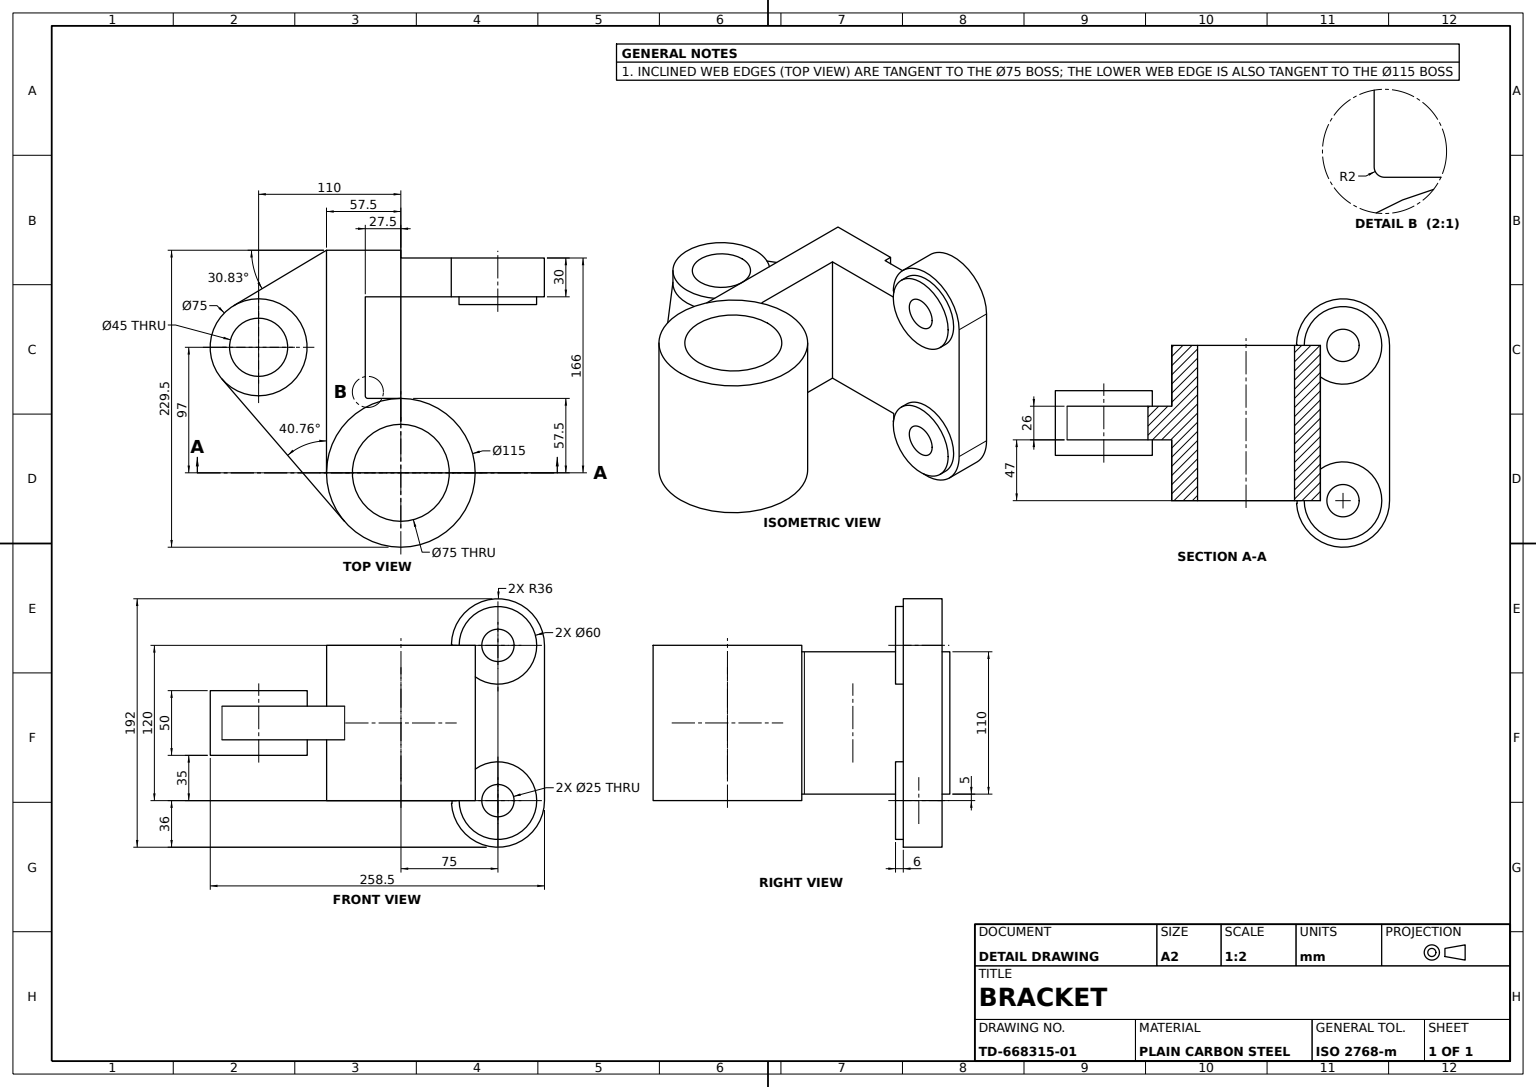
SolidWorks part; units mm, degrees
material "Plain Carbon Steel"
ref_plane "Front Plane" through (0, 0, 0) normal (0, 0, 1) x (1, 0, 0)
ref_plane "Top Plane" through (0, 0, 0) normal (0, 1, 0) x (1, 0, 0)
ref_plane "Right Plane" through (0, 0, 0) normal (1, 0, 0) x (0, 0, -1)
sketch "Base Profile Sketch" plane through (0, 0, 0) normal (0, 0, 1) x (1, 0, 0)
  line L0 (0, 0) -> (-102.5, 0) construction
  line L1 (-36, -60) -> (-102.5, -60)
  line L2 (-102.5, 60) -> (-102.5, -60)
  line L3 (-36, 60) -> (-102.5, 60)
  line L4 (36, 60) -> (36, -60)
  circle A0 centre (0, 60) radius 12.5
  circle A1 centre (0, -60) radius 12.5
  arc A2 (36, 60) -> (-36, 60) centre (0, 60) ccw
  arc A3 (-36, -60) -> (36, -60) centre (0, -60) ccw
  dimension "D3" = 72
  dimension "D4" = 25
  dimension "D5" = 25
  dimension "D6" = 72
  dimension "D1" = 120
  dimension "D2" = 60
  dimension "D7" = 102.5
extrude "Base Body" add sketch "Base Profile Sketch" along normal mid plane 30
sketch "Boss Pad Sketch" plane through (0, 0, 15) normal (0, 0, 1) x (1, 0, 0)
  circle A0 centre (0, -60) radius 30
  circle A1 centre (0, 60) radius 30
  dimension "D1" = 60
  dimension "D2" = 60
extrude "Boss Pad 6mm" add sketch "Boss Pad Sketch" along normal blind 6
sketch "Bore Sketch" plane through (0, 0, -15) normal (0, 0, -1) x (-1, 0, 0)
  circle A0 centre (0, -60) radius 12.5 construction
  circle A1 centre (0, 60) radius 12.5 construction
  circle A6 centre (0, -60) radius 12.5
  circle A7 centre (0, 60) radius 12.5
extrude "Bore Cut" cut sketch "Bore Sketch" against normal through all
sketch "Arm Block Sketch" plane through (0, 0, 0) normal (0, 1, 0) x (1, 0, 0)
  line L0 (0, 0) -> (-75, 0) construction
  line L1 (-75, 15) -> (-75, -151) construction
  line L2 (-102.5, 15) -> (-36, 15) construction
  circle A0 centre (-75, -151) radius 37.5
  circle A1 centre (-75, -151) radius 57.5
  dimension "D3" = 75
  dimension "D4" = 115
  dimension "D1" = 75
  dimension "D2" = 166
extrude "Arm Block" add sketch "Arm Block Sketch" along normal mid plane 120 separate body
sketch "Web Profile Sketch" plane through (0, 0, 0) normal (0, 1, 0) x (1, 0, 0)
  line L0 (0, 0) -> (-132.5, 0) construction
  line L1 (-132.5, -151) -> (-132.5, 21)
  line L2 (-102.5, 15) -> (-36, 15) construction
  line L3 (-132.5, 21) -> (-75, 21)
  line L4 (-75, 21) -> (-75, 15)
  line L5 (-75, 15) -> (-36, 15)
  line L6 (36, 15) -> (-36, 15) construction
  line L7 (-36, -15) -> (-36, 15) construction
  line L8 (-36, 15) -> (-36, -15)
  line L9 (-36, -15) -> (-102.5, -15)
  line L10 (-102.5, -15) -> (-102.5, 15) construction
  line L11 (-102.5, -15) -> (-36, -15) construction
  line L12 (-102.5, -15) -> (-102.5, -91.5)
  line L13 (-100.5, -93.5) -> (-75, -93.5)
  circle A0 centre (-75, -151) radius 57.5 construction
  arc A1 (-102.5, -91.5) -> (-100.5, -93.5) centre (-100.5, -91.5) ccw
  arc A2 (-75, -93.5) -> (-132.5, -151) centre (-75, -151) ccw
  dimension "D4" = 2
  dimension "D1" = 132.5
  dimension "D2" = 6
  dimension "D3" = 57.5
extrude "Web" add sketch "Web Profile Sketch" along normal mid plane 110
sketch "Web Pocket Sketch" plane through (-132.5, 0, 0) normal (-1, 0, 0) x (0, 0, 1)
  line L0 (-21, -55) -> (151, -55) construction
  line L1 (-21, -55) -> (18.3511, -55)
  line L2 (-21, -55) -> (-21, -62.1817)
  line L3 (-21, -62.1817) -> (18.3511, -62.1817)
  line L4 (18.3511, -55) -> (18.3511, -62.1817)
  line L5 (-21, 55) -> (24.7762, 55)
  line L6 (-21, 55) -> (-21, 60.7096)
  line L7 (-21, 60.7096) -> (24.7762, 60.7096)
  line L8 (24.7762, 55) -> (24.7762, 60.7096)
  dimension "D1" = 39.3511
  dimension "D2" = 45.7762
  dimension "D3" = 115.7096
  dimension "D4" = 7.1817
extrude "Web Pocket Cut" cut sketch "Web Pocket Sketch" against normal blind 97
sketch "Mounting Plate Sketch" plane through (0, 0, 0) normal (0, 1, 0) x (1, 0, 0)
  line L0 (-75, -151) -> (-185, -151) construction
  line L1 (-185, -151) -> (-185, 20.4791) construction
  line L2 (-75, 21) -> (-132.5, 21) construction
  circle A0 centre (-185, -54) radius 22.5
  circle A1 centre (-185, -54) radius 37.5
  dimension "D3" = 45
  dimension "D4" = 75
  dimension "D1" = 110
  dimension "D2" = 75
extrude "Mounting Plate" add sketch "Mounting Plate Sketch" along normal mid plane 50 separate body
sketch "Lug Bosses Sketch" plane through (0, 0, 0) normal (0, 1, 0) x (1, 0, 0)
  line L0 (-132.5, 21) -> (-204.2169, -21.7981)
  line L1 (-118.5563, -188.538) -> (-213.4063, -78.4813)
  line L2 (-118.5563, -188.538) -> (-118.5563, 21)
  line L3 (-75, 21) -> (-132.5, 21) construction
  line L4 (-118.5563, 21) -> (-132.5, 21)
  circle A0 centre (-185, -54) radius 37.5 construction
  circle A1 centre (-75, -151) radius 57.5 construction
  arc A2 (-118.5563, -188.538) -> (-118.5563, -113.462) centre (-75, -151) ccw
  arc A3 (-204.2169, -21.7981) -> (-213.4063, -78.4813) centre (-185, -54) ccw
extrude "Lug Bosses" add sketch "Lug Bosses Sketch" along normal mid plane 26 contours L0 A3 L1 L2 L4
sketch "Lug Holes Sketch" plane through (0, -25, 0) normal (0, -1, 0) x (1, 0, 0)
  circle A0 centre (-185, 54) radius 22.5 construction
  circle A1 centre (-185, 54) radius 22.5
extrude "Lug Holes Cut" cut sketch "Lug Holes Sketch" against normal through all
